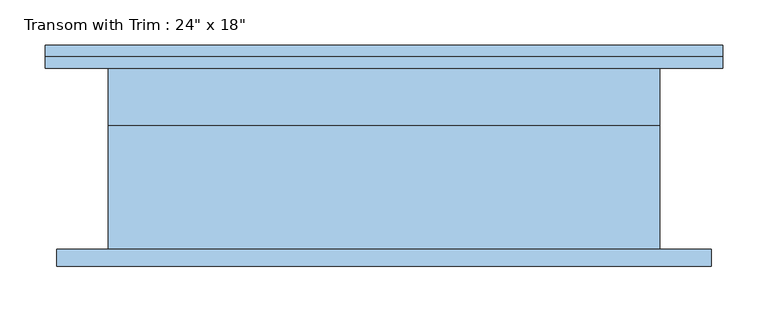
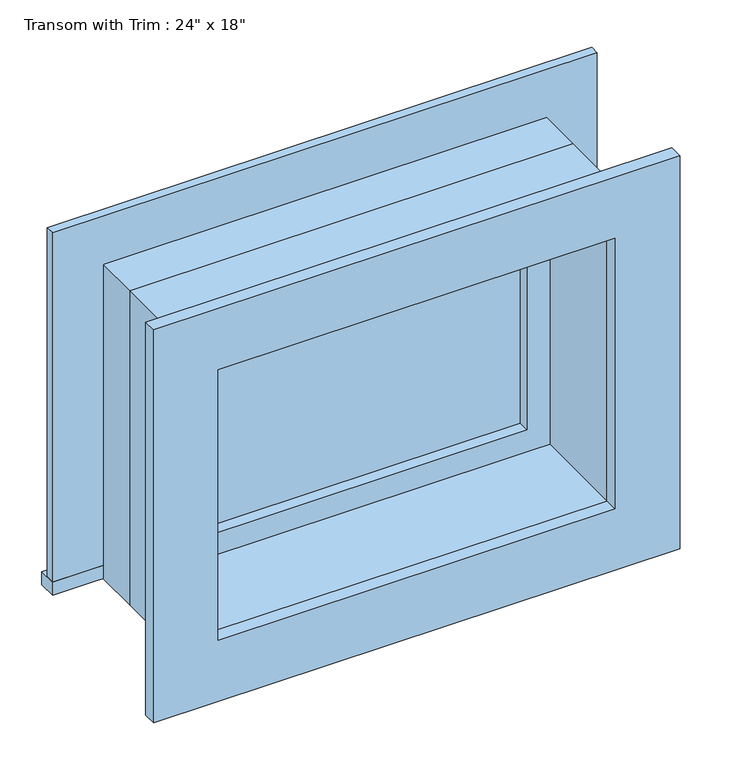
"""IFC4 building model written with IfcOpenShell, lengths in millimetres: window geometry."""

from ifc_helpers import new_model, si_unit, frame, origin, place, context, project, spatial, polyline, outline, extrude, source, transform, mapped, element, save


def window_372a270f(model_context):
    return source(origin(), model_context, "Body", "SweptSolid", [
        extrude(outline(polyline([(-412.75, 125.4), (336.55, 125.4), (336.55, 100.0), (-412.75, 100.0), (-412.75, 125.4)])), frame((0.0, 0.0, 2159.0), z_axis=(0.0, 0.0, 1.0), x_axis=(1.0, 0.0, 0.0)), (0.0, 0.0, 1.0), 19.05),
        extrude(outline(polyline([(2597.15, -323.85), (2597.15, 247.65), (2178.05, 247.65), (2178.05, 336.55), (2686.05, 336.55), (2686.05, -412.75), (2178.05, -412.75), (2178.05, -323.85), (2597.15, -323.85)])), frame((0.0, 100.0, 0.0), z_axis=(0.0, 1.0, 0.0), x_axis=(0.0, 0.0, 1.0)), (0.0, 0.0, 1.0), 12.7),
        extrude(outline(polyline([(2673.35, 323.85), (2673.35, -400.05), (2101.85, -400.05), (2101.85, 323.85), (2673.35, 323.85)]), holes=[polyline([(2584.45, 234.95), (2190.75, 234.95), (2190.75, -311.15), (2584.45, -311.15), (2584.45, 234.95)])]), frame((0.0, -119.05, 0.0), z_axis=(0.0, 1.0, 0.0), x_axis=(0.0, 0.0, 1.0)), (0.0, 0.0, 1.0), 19.05),
        extrude(outline(polyline([(203.2, 52.375), (-279.4, 52.375), (-279.4, 65.075), (203.2, 65.075), (203.2, 52.375)])), frame((0.0, 0.0, 2222.5), z_axis=(0.0, 0.0, 1.0), x_axis=(1.0, 0.0, 0.0)), (0.0, 0.0, 1.0), 330.2),
        extrude(outline(polyline([(2597.15, -323.85), (2178.05, -323.85), (2178.05, 247.65), (2597.15, 247.65), (2597.15, -323.85)]), holes=[polyline([(2552.7, -279.4), (2552.7, 203.2), (2222.5, 203.2), (2222.5, -279.4), (2552.7, -279.4)])]), frame((0.0, 36.5, 0.0), z_axis=(0.0, 1.0, 0.0), x_axis=(0.0, 0.0, 1.0)), (0.0, 0.0, 1.0), 44.45),
        extrude(outline(polyline([(2616.2, -342.9), (2159.0, -342.9), (2159.0, 266.7), (2616.2, 266.7), (2616.2, -342.9)]), holes=[polyline([(2584.45, -311.15), (2584.45, 234.95), (2190.75, 234.95), (2190.75, -311.15), (2584.45, -311.15)])]), frame((0.0, -100.0, 0.0), z_axis=(0.0, 1.0, 0.0), x_axis=(0.0, 0.0, 1.0)), (0.0, 0.0, 1.0), 136.5),
        extrude(outline(polyline([(2616.2, 266.7), (2616.2, -342.9), (2159.0, -342.9), (2159.0, 266.7), (2616.2, 266.7)]), holes=[polyline([(2597.15, 247.65), (2178.05, 247.65), (2178.05, -323.85), (2597.15, -323.85), (2597.15, 247.65)])]), frame((0.0, 36.5, 0.0), z_axis=(0.0, 1.0, 0.0), x_axis=(0.0, 0.0, 1.0)), (0.0, 0.0, 1.0), 63.5),
    ])


if __name__ == "__main__":
    model = new_model("IFC4")
    model_context = context("Model", 3, world=origin())
    ifc_project = project(units=[si_unit("LENGTHUNIT", "METRE", prefix="MILLI")], contexts=[model_context])
    site = spatial("IfcSite", under=ifc_project)
    building = spatial("IfcBuilding", under=site)
    placement = place(None, origin())
    window_shape = window_372a270f(model_context)
    element("IfcWindow", 1, ObjectType="Transom with Trim : 24\" x 18\"", at=placement, inside=building, context=model_context, shape_type="MappedRepresentation", body=[
        mapped(window_shape, transform((0.0, 0.0, 0.0), x_axis=(1.0, 0.0, 0.0), y_axis=(0.0, 1.0, 0.0), z_axis=(0.0, 0.0, 1.0))),
    ])
    save(model, "model.ifc")

# Revit data of these elements
# Type "Transom with Trim : 24\" x 18\""
#   Type Mark = "30"
#   Construction Type Id = "GSP4R"
#   Assembly Code = "B2020100"
#   Analytic Construction = "1/8 in Pilkington single glazing"
#   Visual Light Transmittance = 0.9
#   Solar Heat Gain Coefficient = 0.78
#   Heat Transfer Coefficient (U) = 3.6886 W/(m²·K)
#   Height = 1' - 6"
#   Default Sill Height = 7' - 1"
#   Trim Projection - Ext. = 0' - 0 1/2"
#   Trim Projection - Int. = 0' - 0 3/4"
#   Trim Width - Exterior = 0' - 3 1/2"
#   Trim Width - Interior = 0' - 3 1/2"
#   Width = 2' - 0"
#   Window Inset = 0' - 0 3/4"
#   Define Thermal Properties by = 1
#   Glass Pane Material = Glass
#   Sash Material = Sash
#   Trim Exterior Material = Trim
#   Trim Interior Material = Trim
#   Wall Closure = (empty or 0)
# Element 1 (IfcWindow, "Transom with Trim : 24\" x 18\"")
#   Materials on its faces: "Sash", "Trim", "Glass"
# Materials
#   "Glass": class "Glass", colour RGB 218 227 224, transparency 0.85, Description = "Soda Lime Glass", Cost = 0
#   "Sash": class "Wood", colour RGB 136 99 55, transparency 0
#   "Trim": class "Wood", colour RGB 224 178 126, transparency 0
